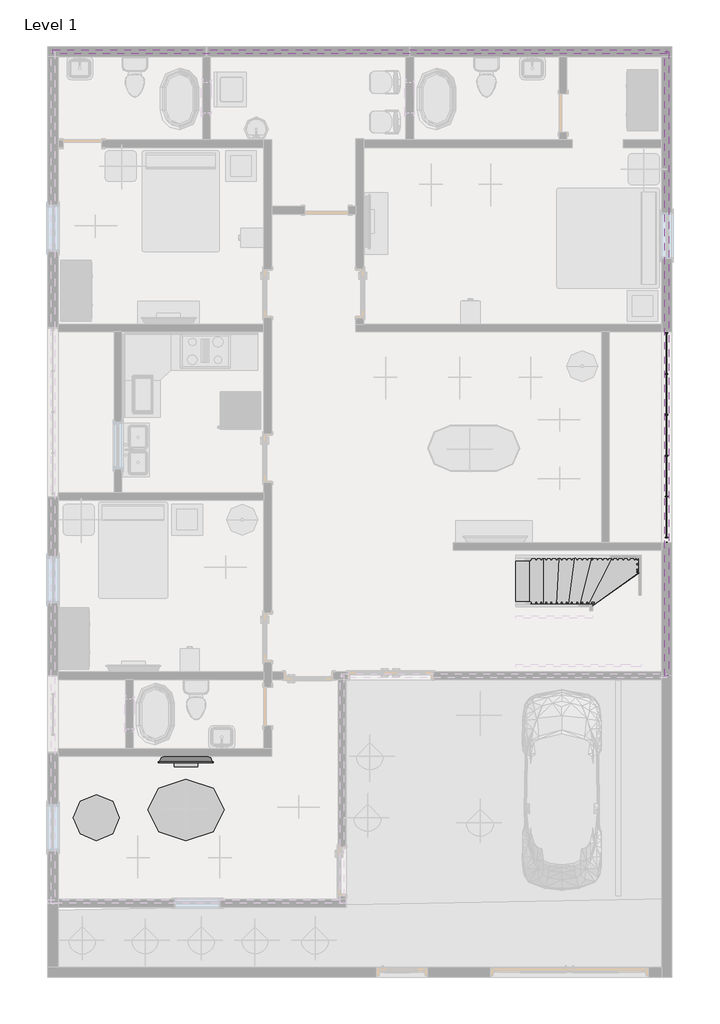
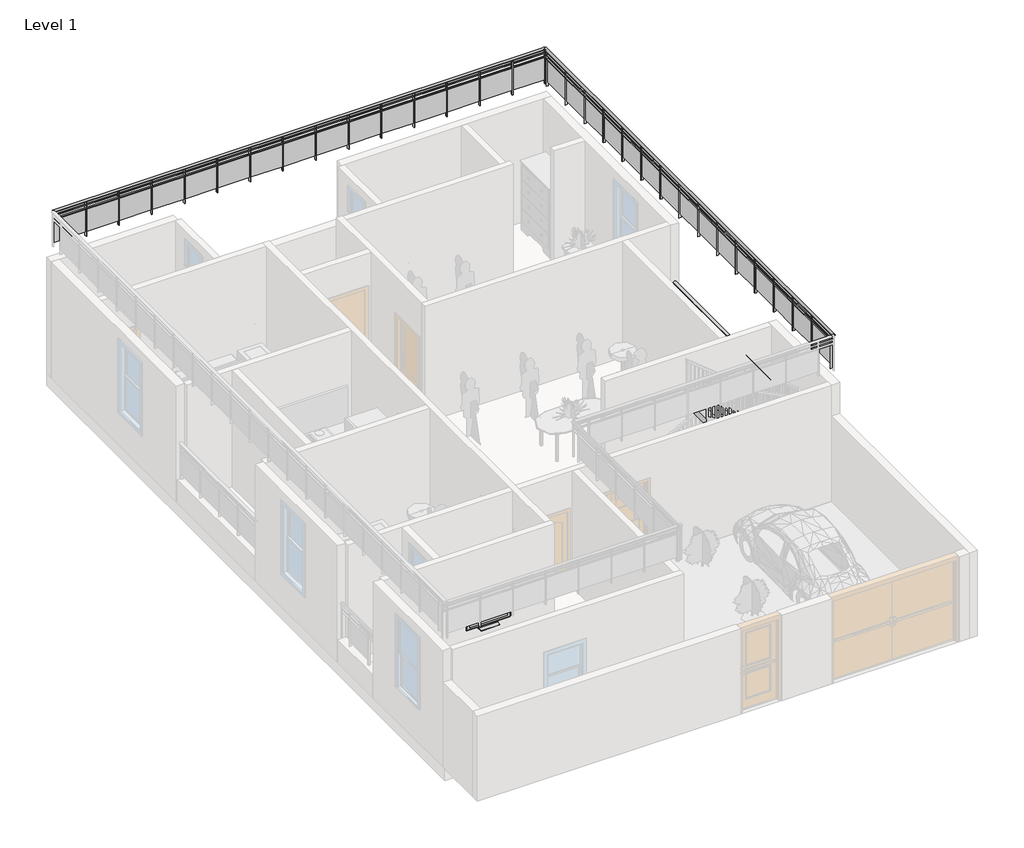
# One storey, part 5 of 6: 3 furniture elements, 3 railings, 1 stair flight.
"""IFC4 building model written with IfcOpenShell, lengths in millimetres."""

from ifc_helpers import new_model, si_unit, point, frame, origin, place, context, project, spatial, polyline, ellipse_curve, trimmed, outline, extrude, transform, mapped, element, save
from ifc_brep_helpers import plane_surface, extruded_surface, advanced_brep
from components import furniture_7a3aaa4f, furniture_905aceb5, furniture_743965d2, stair_flight_813748e6

model = new_model("IFC4")

# Units and contexts
model_context = context("Model", 3, world=origin())
ifc_project = project(units=[si_unit("LENGTHUNIT", "METRE", prefix="MILLI")], contexts=[model_context])

# Site, building, storey
site = spatial("IfcSite", under=ifc_project)
building = spatial("IfcBuilding", under=site)
storey = spatial("IfcBuildingStorey", under=building, Name="Level 1", Elevation=0.0)

# Furniture
placement = place(None, origin())
furniture_shape = furniture_7a3aaa4f(model_context)
element("IfcFurniture", 1, ObjectType="TV - Flat Screen : 42\"", at=placement, inside=storey, context=model_context, shape_type="MappedRepresentation", body=[
    mapped(furniture_shape, transform((-11860.0396044, -302.3114474, 1041.4), x_axis=(1.0, 0.0, 0.0), y_axis=(0.0, 1.0, 0.0), z_axis=(0.0, 0.0, 1.0))),
])
furniture_2_shape = furniture_905aceb5(model_context)
element("IfcFurniture", 2, ObjectType="Table-Dining Round w Chairs : 36\" Diameter", at=placement, inside=storey, context=model_context, shape_type="MappedRepresentation", body=[
    mapped(furniture_2_shape, transform((-13745.6660857, -1278.0941352, 0.0), x_axis=(1.0, 0.0, 0.0), y_axis=(0.0, 1.0, 0.0), z_axis=(0.0, 0.0, 1.0))),
])
furniture_3_shape = furniture_743965d2(model_context)
element("IfcFurniture", 3, ObjectType="Table-Ellipse : 60\" x 48\"", at=placement, inside=storey, context=model_context, shape_type="MappedRepresentation", body=[
    mapped(furniture_3_shape, transform((-11863.9841185, -1310.5728237, 0.0), x_axis=(1.0, 0.0, 0.0), y_axis=(0.0, 1.0, 0.0), z_axis=(0.0, 0.0, 1.0))),
])

# Railings
element("IfcRailing", 4, ObjectType="Glass Panel - Bottom Fill", at=placement, inside=storey, context=model_context, shape_type="SolidModel", body=[
    advanced_brep(
    [(-2351.6841185, 3998.0271763, 1524.0), (-2275.4841185, 3998.0271763, 1524.0), (-2351.6841185, 8265.2271763, 1524.0), (-2275.4841185, 8265.2271763, 1524.0)],
    [
        (0, 1, ellipse_curve(frame((-2313.5841185, 3998.0271763, 1524.0), z_axis=(0.0, -1.0, 0.0), x_axis=(1.0, 0.0, 0.0)), 38.1, 28.575)),
        (1, 0, ellipse_curve(frame((-2313.5841185, 3998.0271763, 1524.0), z_axis=(0.0, -1.0, 0.0), x_axis=(1.0, 0.0, 0.0)), 38.1, 28.575)),
        (2, 3, ellipse_curve(frame((-2313.5841185, 8265.2271763, 1524.0), z_axis=(0.0, 1.0, 0.0), x_axis=(1.0, 0.0, 0.0)), 38.1, 28.575)),
        (3, 2, ellipse_curve(frame((-2313.5841185, 8265.2271763, 1524.0), z_axis=(0.0, 1.0, 0.0), x_axis=(1.0, 0.0, 0.0)), 38.1, 28.575)),
        (0, 2),
        (3, 1),
    ],
    [
        plane_surface(frame((-2313.5841185, 3998.0271763, 1524.0), z_axis=(0.0, -1.0, 0.0), x_axis=(0.0, 0.0, 1.0))),
        plane_surface(frame((-2313.5841185, 8265.2271763, 1524.0), z_axis=(0.0, 1.0, 0.0), x_axis=(0.0, 0.0, 1.0))),
        extruded_surface(trimmed(ellipse_curve(frame((-2313.5841185, 8265.2271763, 1524.0), z_axis=(0.0, -1.0, 0.0), x_axis=(1.0, 0.0, 0.0)), 38.1, 28.575), [point((-2351.6841185, 8265.2271763, 1524.0))], [point((-2275.4841185, 8265.2271763, 1524.0))], True, "CARTESIAN"), (0.0, -4267.200000000001, 0.0), 4267.200000000001),
        extruded_surface(trimmed(ellipse_curve(frame((-2313.5841185, 8265.2271763, 1524.0), z_axis=(0.0, -1.0, 0.0), x_axis=(1.0, 0.0, 0.0)), 38.1, 28.575), [point((-2275.4841185, 8265.2271763, 1524.0))], [point((-2351.6841185, 8265.2271763, 1524.0))], True, "CARTESIAN"), (0.0, -4267.200000000001, 0.0), 4267.200000000001),
    ],
    [
        (0, [[1, 2]]),
        (1, [[3, 4]]),
        (2, [[-1, 5, -4, 6]]),
        (3, [[-2, -6, -3, -5]]),
    ],
),
    extrude(outline(polyline([(-2300.8841185, 3998.0271763), (-2326.2841185, 3998.0271763), (-2326.2841185, 8265.2271763), (-2300.8841185, 8265.2271763), (-2300.8841185, 3998.0271763)])), frame((0.0, 0.0, 1409.7), z_axis=(0.0, 0.0, 1.0), x_axis=(1.0, 0.0, 0.0)), (0.0, 0.0, 1.0), 25.4),
    extrude(outline(polyline([(-2300.8841185, 3998.0271763), (-2326.2841185, 3998.0271763), (-2326.2841185, 8265.2271763), (-2300.8841185, 8265.2271763), (-2300.8841185, 3998.0271763)])), frame((0.0, 0.0, 1308.1), z_axis=(0.0, 0.0, 1.0), x_axis=(1.0, 0.0, 0.0)), (0.0, 0.0, 1.0), 25.4),
    extrude(outline(polyline([(-2288.1841185, 8157.2771763), (-2338.9841185, 8157.2771763), (-2338.9841185, 8169.9771763), (-2288.1841185, 8169.9771763), (-2288.1841185, 8157.2771763)])), frame((0.0, 0.0, 609.6), z_axis=(0.0, 0.0, 1.0), x_axis=(1.0, 0.0, 0.0)), (0.0, 0.0, 1.0), 885.6788223),
    extrude(outline(polyline([(-2320.1192755, 7350.8271763), (-2320.1192755, 8163.6271763), (-2313.7692755, 8163.6271763), (-2313.7692755, 7350.8271763), (-2320.1192755, 7350.8271763)])), frame((0.0, 0.0, 711.2), z_axis=(0.0, 0.0, 1.0), x_axis=(1.0, 0.0, 0.0)), (0.0, 0.0, 1.0), 596.9),
    extrude(outline(polyline([(-2288.1841185, 7344.4771763), (-2338.9841185, 7344.4771763), (-2338.9841185, 7357.1771763), (-2288.1841185, 7357.1771763), (-2288.1841185, 7344.4771763)])), frame((0.0, 0.0, 609.6), z_axis=(0.0, 0.0, 1.0), x_axis=(1.0, 0.0, 0.0)), (0.0, 0.0, 1.0), 885.6788223),
    extrude(outline(polyline([(-2320.1192755, 6538.0271763), (-2320.1192755, 7350.8271763), (-2313.7692755, 7350.8271763), (-2313.7692755, 6538.0271763), (-2320.1192755, 6538.0271763)])), frame((0.0, 0.0, 711.2), z_axis=(0.0, 0.0, 1.0), x_axis=(1.0, 0.0, 0.0)), (0.0, 0.0, 1.0), 596.9),
    extrude(outline(polyline([(-2288.1841185, 6531.6771763), (-2338.9841185, 6531.6771763), (-2338.9841185, 6544.3771763), (-2288.1841185, 6544.3771763), (-2288.1841185, 6531.6771763)])), frame((0.0, 0.0, 609.6), z_axis=(0.0, 0.0, 1.0), x_axis=(1.0, 0.0, 0.0)), (0.0, 0.0, 1.0), 885.6788223),
    extrude(outline(polyline([(-2320.1192755, 5725.2271763), (-2320.1192755, 6538.0271763), (-2313.7692755, 6538.0271763), (-2313.7692755, 5725.2271763), (-2320.1192755, 5725.2271763)])), frame((0.0, 0.0, 711.2), z_axis=(0.0, 0.0, 1.0), x_axis=(1.0, 0.0, 0.0)), (0.0, 0.0, 1.0), 596.9),
    extrude(outline(polyline([(-2288.1841185, 5718.8771763), (-2338.9841185, 5718.8771763), (-2338.9841185, 5731.5771763), (-2288.1841185, 5731.5771763), (-2288.1841185, 5718.8771763)])), frame((0.0, 0.0, 609.6), z_axis=(0.0, 0.0, 1.0), x_axis=(1.0, 0.0, 0.0)), (0.0, 0.0, 1.0), 885.6788223),
    extrude(outline(polyline([(-2320.1192755, 4912.4271763), (-2320.1192755, 5725.2271763), (-2313.7692755, 5725.2271763), (-2313.7692755, 4912.4271763), (-2320.1192755, 4912.4271763)])), frame((0.0, 0.0, 711.2), z_axis=(0.0, 0.0, 1.0), x_axis=(1.0, 0.0, 0.0)), (0.0, 0.0, 1.0), 596.9),
    extrude(outline(polyline([(-2288.1841185, 4906.0771763), (-2338.9841185, 4906.0771763), (-2338.9841185, 4918.7771763), (-2288.1841185, 4918.7771763), (-2288.1841185, 4906.0771763)])), frame((0.0, 0.0, 609.6), z_axis=(0.0, 0.0, 1.0), x_axis=(1.0, 0.0, 0.0)), (0.0, 0.0, 1.0), 885.6788223),
    extrude(outline(polyline([(-2320.1192755, 4099.6271763), (-2320.1192755, 4912.4271763), (-2313.7692755, 4912.4271763), (-2313.7692755, 4099.6271763), (-2320.1192755, 4099.6271763)])), frame((0.0, 0.0, 711.2), z_axis=(0.0, 0.0, 1.0), x_axis=(1.0, 0.0, 0.0)), (0.0, 0.0, 1.0), 596.9),
    extrude(outline(polyline([(-2288.1841185, 4093.2771763), (-2338.9841185, 4093.2771763), (-2338.9841185, 4105.9771763), (-2288.1841185, 4105.9771763), (-2288.1841185, 4093.2771763)])), frame((0.0, 0.0, 609.6), z_axis=(0.0, 0.0, 1.0), x_axis=(1.0, 0.0, 0.0)), (0.0, 0.0, 1.0), 885.6788223),
    extrude(outline(polyline([(-2304.0591185, 8252.5271763), (-2323.1091185, 8252.5271763), (-2323.1091185, 8271.5771763), (-2304.0591185, 8271.5771763), (-2304.0591185, 8252.5271763)])), frame((0.0, 0.0, 609.6), z_axis=(0.0, 0.0, 1.0), x_axis=(1.0, 0.0, 0.0)), (0.0, 0.0, 1.0), 885.6788223),
    extrude(outline(polyline([(-2304.0591185, 3991.6771763), (-2323.1091185, 3991.6771763), (-2323.1091185, 4010.7271763), (-2304.0591185, 4010.7271763), (-2304.0591185, 3991.6771763)])), frame((0.0, 0.0, 609.6), z_axis=(0.0, 0.0, 1.0), x_axis=(1.0, 0.0, 0.0)), (0.0, 0.0, 1.0), 885.6788223),
])
element("IfcRailing", 5, ObjectType="Glass Panel - Bottom Fill", at=placement, inside=storey, context=model_context, shape_type="SolidModel", body=[
    advanced_brep(
    [(-14505.5841185, 13789.7271763, 4267.2), (-14505.5841185, 13713.5271763, 4267.2), (-2313.5841185, 13789.7271763, 4267.2), (-2313.5841185, 13713.5271763, 4267.2)],
    [
        (0, 1, ellipse_curve(frame((-14505.5841185, 13751.6271763, 4267.2), z_axis=(-1.0, 0.0, 0.0), x_axis=(0.0, -1.0, 0.0)), 38.1, 28.575)),
        (1, 0, ellipse_curve(frame((-14505.5841185, 13751.6271763, 4267.2), z_axis=(-1.0, 0.0, 0.0), x_axis=(0.0, -1.0, 0.0)), 38.1, 28.575)),
        (2, 3, ellipse_curve(frame((-2313.5841185, 13751.6271763, 4267.2), z_axis=(1.0, 0.0, 0.0), x_axis=(0.0, -1.0, 0.0)), 38.1, 28.575)),
        (3, 2, ellipse_curve(frame((-2313.5841185, 13751.6271763, 4267.2), z_axis=(1.0, 0.0, 0.0), x_axis=(0.0, -1.0, 0.0)), 38.1, 28.575)),
        (0, 2),
        (3, 1),
    ],
    [
        plane_surface(frame((-14505.5841185, 13751.6271763, 4267.2), z_axis=(-1.0, 0.0, 0.0), x_axis=(0.0, 1.0, 0.0))),
        plane_surface(frame((-2313.5841185, 13751.6271763, 4267.2), z_axis=(1.0, 0.0, 0.0), x_axis=(0.0, 1.0, 0.0))),
        extruded_surface(trimmed(ellipse_curve(frame((-2313.5841185, 13751.6271763, 4267.2), z_axis=(-1.0, 0.0, 0.0), x_axis=(0.0, -1.0, 0.0)), 38.1, 28.575), [point((-2313.5841185, 13789.7271763, 4267.2))], [point((-2313.5841185, 13713.5271763, 4267.2))], True, "CARTESIAN"), (-12192.0, 0.0, 0.0), 12192.0),
        extruded_surface(trimmed(ellipse_curve(frame((-2313.5841185, 13751.6271763, 4267.2), z_axis=(-1.0, 0.0, 0.0), x_axis=(0.0, -1.0, 0.0)), 38.1, 28.575), [point((-2313.5841185, 13713.5271763, 4267.2))], [point((-2313.5841185, 13789.7271763, 4267.2))], True, "CARTESIAN"), (-12192.0, 0.0, 0.0), 12192.0),
    ],
    [
        (0, [[1, 2]]),
        (1, [[3, 4]]),
        (2, [[-1, 5, -4, 6]]),
        (3, [[-2, -6, -3, -5]]),
    ],
),
    extrude(outline(polyline([(-14505.5841185, 13738.9271763), (-14505.5841185, 13764.3271763), (-2313.5841185, 13764.3271763), (-2313.5841185, 13738.9271763), (-14505.5841185, 13738.9271763)])), frame((0.0, 0.0, 4152.9), z_axis=(0.0, 0.0, 1.0), x_axis=(1.0, 0.0, 0.0)), (0.0, 0.0, 1.0), 25.4),
    extrude(outline(polyline([(-14505.5841185, 13738.9271763), (-14505.5841185, 13764.3271763), (-2313.5841185, 13764.3271763), (-2313.5841185, 13738.9271763), (-14505.5841185, 13738.9271763)])), frame((0.0, 0.0, 4051.3), z_axis=(0.0, 0.0, 1.0), x_axis=(1.0, 0.0, 0.0)), (0.0, 0.0, 1.0), 25.4),
    extrude(outline(polyline([(-3126.3841185, 13758.1623333), (-2313.5841185, 13758.1623333), (-2313.5841185, 13751.8123333), (-3126.3841185, 13751.8123333), (-3126.3841185, 13758.1623333)])), frame((0.0, 0.0, 3454.4), z_axis=(0.0, 0.0, 1.0), x_axis=(1.0, 0.0, 0.0)), (0.0, 0.0, 1.0), 596.9),
    extrude(outline(polyline([(-3132.7341185, 13726.2271763), (-3132.7341185, 13777.0271763), (-3120.0341185, 13777.0271763), (-3120.0341185, 13726.2271763), (-3132.7341185, 13726.2271763)])), frame((0.0, 0.0, 3352.8), z_axis=(0.0, 0.0, 1.0), x_axis=(1.0, 0.0, 0.0)), (0.0, 0.0, 1.0), 885.6788223),
    extrude(outline(polyline([(-3939.1841185, 13758.1623333), (-3126.3841185, 13758.1623333), (-3126.3841185, 13751.8123333), (-3939.1841185, 13751.8123333), (-3939.1841185, 13758.1623333)])), frame((0.0, 0.0, 3454.4), z_axis=(0.0, 0.0, 1.0), x_axis=(1.0, 0.0, 0.0)), (0.0, 0.0, 1.0), 596.9),
    extrude(outline(polyline([(-3945.5341185, 13726.2271763), (-3945.5341185, 13777.0271763), (-3932.8341185, 13777.0271763), (-3932.8341185, 13726.2271763), (-3945.5341185, 13726.2271763)])), frame((0.0, 0.0, 3352.8), z_axis=(0.0, 0.0, 1.0), x_axis=(1.0, 0.0, 0.0)), (0.0, 0.0, 1.0), 885.6788223),
    extrude(outline(polyline([(-4751.9841185, 13758.1623333), (-3939.1841185, 13758.1623333), (-3939.1841185, 13751.8123333), (-4751.9841185, 13751.8123333), (-4751.9841185, 13758.1623333)])), frame((0.0, 0.0, 3454.4), z_axis=(0.0, 0.0, 1.0), x_axis=(1.0, 0.0, 0.0)), (0.0, 0.0, 1.0), 596.9),
    extrude(outline(polyline([(-4758.3341185, 13726.2271763), (-4758.3341185, 13777.0271763), (-4745.6341185, 13777.0271763), (-4745.6341185, 13726.2271763), (-4758.3341185, 13726.2271763)])), frame((0.0, 0.0, 3352.8), z_axis=(0.0, 0.0, 1.0), x_axis=(1.0, 0.0, 0.0)), (0.0, 0.0, 1.0), 885.6788223),
    extrude(outline(polyline([(-5564.7841185, 13758.1623333), (-4751.9841185, 13758.1623333), (-4751.9841185, 13751.8123333), (-5564.7841185, 13751.8123333), (-5564.7841185, 13758.1623333)])), frame((0.0, 0.0, 3454.4), z_axis=(0.0, 0.0, 1.0), x_axis=(1.0, 0.0, 0.0)), (0.0, 0.0, 1.0), 596.9),
    extrude(outline(polyline([(-5571.1341185, 13726.2271763), (-5571.1341185, 13777.0271763), (-5558.4341185, 13777.0271763), (-5558.4341185, 13726.2271763), (-5571.1341185, 13726.2271763)])), frame((0.0, 0.0, 3352.8), z_axis=(0.0, 0.0, 1.0), x_axis=(1.0, 0.0, 0.0)), (0.0, 0.0, 1.0), 885.6788223),
    extrude(outline(polyline([(-6377.5841185, 13758.1623333), (-5564.7841185, 13758.1623333), (-5564.7841185, 13751.8123333), (-6377.5841185, 13751.8123333), (-6377.5841185, 13758.1623333)])), frame((0.0, 0.0, 3454.4), z_axis=(0.0, 0.0, 1.0), x_axis=(1.0, 0.0, 0.0)), (0.0, 0.0, 1.0), 596.9),
    extrude(outline(polyline([(-6383.9341185, 13726.2271763), (-6383.9341185, 13777.0271763), (-6371.2341185, 13777.0271763), (-6371.2341185, 13726.2271763), (-6383.9341185, 13726.2271763)])), frame((0.0, 0.0, 3352.8), z_axis=(0.0, 0.0, 1.0), x_axis=(1.0, 0.0, 0.0)), (0.0, 0.0, 1.0), 885.6788223),
    extrude(outline(polyline([(-7190.3841185, 13758.1623333), (-6377.5841185, 13758.1623333), (-6377.5841185, 13751.8123333), (-7190.3841185, 13751.8123333), (-7190.3841185, 13758.1623333)])), frame((0.0, 0.0, 3454.4), z_axis=(0.0, 0.0, 1.0), x_axis=(1.0, 0.0, 0.0)), (0.0, 0.0, 1.0), 596.9),
    extrude(outline(polyline([(-7196.7341185, 13726.2271763), (-7196.7341185, 13777.0271763), (-7184.0341185, 13777.0271763), (-7184.0341185, 13726.2271763), (-7196.7341185, 13726.2271763)])), frame((0.0, 0.0, 3352.8), z_axis=(0.0, 0.0, 1.0), x_axis=(1.0, 0.0, 0.0)), (0.0, 0.0, 1.0), 885.6788223),
    extrude(outline(polyline([(-8003.1841185, 13758.1623333), (-7190.3841185, 13758.1623333), (-7190.3841185, 13751.8123333), (-8003.1841185, 13751.8123333), (-8003.1841185, 13758.1623333)])), frame((0.0, 0.0, 3454.4), z_axis=(0.0, 0.0, 1.0), x_axis=(1.0, 0.0, 0.0)), (0.0, 0.0, 1.0), 596.9),
    extrude(outline(polyline([(-8009.5341185, 13726.2271763), (-8009.5341185, 13777.0271763), (-7996.8341185, 13777.0271763), (-7996.8341185, 13726.2271763), (-8009.5341185, 13726.2271763)])), frame((0.0, 0.0, 3352.8), z_axis=(0.0, 0.0, 1.0), x_axis=(1.0, 0.0, 0.0)), (0.0, 0.0, 1.0), 885.6788223),
    extrude(outline(polyline([(-8815.9841185, 13758.1623333), (-8003.1841185, 13758.1623333), (-8003.1841185, 13751.8123333), (-8815.9841185, 13751.8123333), (-8815.9841185, 13758.1623333)])), frame((0.0, 0.0, 3454.4), z_axis=(0.0, 0.0, 1.0), x_axis=(1.0, 0.0, 0.0)), (0.0, 0.0, 1.0), 596.9),
    extrude(outline(polyline([(-8822.3341185, 13726.2271763), (-8822.3341185, 13777.0271763), (-8809.6341185, 13777.0271763), (-8809.6341185, 13726.2271763), (-8822.3341185, 13726.2271763)])), frame((0.0, 0.0, 3352.8), z_axis=(0.0, 0.0, 1.0), x_axis=(1.0, 0.0, 0.0)), (0.0, 0.0, 1.0), 885.6788223),
    extrude(outline(polyline([(-9628.7841185, 13758.1623333), (-8815.9841185, 13758.1623333), (-8815.9841185, 13751.8123333), (-9628.7841185, 13751.8123333), (-9628.7841185, 13758.1623333)])), frame((0.0, 0.0, 3454.4), z_axis=(0.0, 0.0, 1.0), x_axis=(1.0, 0.0, 0.0)), (0.0, 0.0, 1.0), 596.9),
    extrude(outline(polyline([(-9635.1341185, 13726.2271763), (-9635.1341185, 13777.0271763), (-9622.4341185, 13777.0271763), (-9622.4341185, 13726.2271763), (-9635.1341185, 13726.2271763)])), frame((0.0, 0.0, 3352.8), z_axis=(0.0, 0.0, 1.0), x_axis=(1.0, 0.0, 0.0)), (0.0, 0.0, 1.0), 885.6788223),
    extrude(outline(polyline([(-10441.5841185, 13758.1623333), (-9628.7841185, 13758.1623333), (-9628.7841185, 13751.8123333), (-10441.5841185, 13751.8123333), (-10441.5841185, 13758.1623333)])), frame((0.0, 0.0, 3454.4), z_axis=(0.0, 0.0, 1.0), x_axis=(1.0, 0.0, 0.0)), (0.0, 0.0, 1.0), 596.9),
    extrude(outline(polyline([(-10447.9341185, 13726.2271763), (-10447.9341185, 13777.0271763), (-10435.2341185, 13777.0271763), (-10435.2341185, 13726.2271763), (-10447.9341185, 13726.2271763)])), frame((0.0, 0.0, 3352.8), z_axis=(0.0, 0.0, 1.0), x_axis=(1.0, 0.0, 0.0)), (0.0, 0.0, 1.0), 885.6788223),
    extrude(outline(polyline([(-11254.3841185, 13758.1623333), (-10441.5841185, 13758.1623333), (-10441.5841185, 13751.8123333), (-11254.3841185, 13751.8123333), (-11254.3841185, 13758.1623333)])), frame((0.0, 0.0, 3454.4), z_axis=(0.0, 0.0, 1.0), x_axis=(1.0, 0.0, 0.0)), (0.0, 0.0, 1.0), 596.9),
    extrude(outline(polyline([(-11260.7341185, 13726.2271763), (-11260.7341185, 13777.0271763), (-11248.0341185, 13777.0271763), (-11248.0341185, 13726.2271763), (-11260.7341185, 13726.2271763)])), frame((0.0, 0.0, 3352.8), z_axis=(0.0, 0.0, 1.0), x_axis=(1.0, 0.0, 0.0)), (0.0, 0.0, 1.0), 885.6788223),
    extrude(outline(polyline([(-12067.1841185, 13758.1623333), (-11254.3841185, 13758.1623333), (-11254.3841185, 13751.8123333), (-12067.1841185, 13751.8123333), (-12067.1841185, 13758.1623333)])), frame((0.0, 0.0, 3454.4), z_axis=(0.0, 0.0, 1.0), x_axis=(1.0, 0.0, 0.0)), (0.0, 0.0, 1.0), 596.9),
    extrude(outline(polyline([(-12073.5341185, 13726.2271763), (-12073.5341185, 13777.0271763), (-12060.8341185, 13777.0271763), (-12060.8341185, 13726.2271763), (-12073.5341185, 13726.2271763)])), frame((0.0, 0.0, 3352.8), z_axis=(0.0, 0.0, 1.0), x_axis=(1.0, 0.0, 0.0)), (0.0, 0.0, 1.0), 885.6788223),
    extrude(outline(polyline([(-12879.9841185, 13758.1623333), (-12067.1841185, 13758.1623333), (-12067.1841185, 13751.8123333), (-12879.9841185, 13751.8123333), (-12879.9841185, 13758.1623333)])), frame((0.0, 0.0, 3454.4), z_axis=(0.0, 0.0, 1.0), x_axis=(1.0, 0.0, 0.0)), (0.0, 0.0, 1.0), 596.9),
    extrude(outline(polyline([(-12886.3341185, 13726.2271763), (-12886.3341185, 13777.0271763), (-12873.6341185, 13777.0271763), (-12873.6341185, 13726.2271763), (-12886.3341185, 13726.2271763)])), frame((0.0, 0.0, 3352.8), z_axis=(0.0, 0.0, 1.0), x_axis=(1.0, 0.0, 0.0)), (0.0, 0.0, 1.0), 885.6788223),
    extrude(outline(polyline([(-13692.7841185, 13758.1623333), (-12879.9841185, 13758.1623333), (-12879.9841185, 13751.8123333), (-13692.7841185, 13751.8123333), (-13692.7841185, 13758.1623333)])), frame((0.0, 0.0, 3454.4), z_axis=(0.0, 0.0, 1.0), x_axis=(1.0, 0.0, 0.0)), (0.0, 0.0, 1.0), 596.9),
    extrude(outline(polyline([(-13699.1341185, 13726.2271763), (-13699.1341185, 13777.0271763), (-13686.4341185, 13777.0271763), (-13686.4341185, 13726.2271763), (-13699.1341185, 13726.2271763)])), frame((0.0, 0.0, 3352.8), z_axis=(0.0, 0.0, 1.0), x_axis=(1.0, 0.0, 0.0)), (0.0, 0.0, 1.0), 885.6788223),
    extrude(outline(polyline([(-14505.5841185, 13758.1623333), (-13692.7841185, 13758.1623333), (-13692.7841185, 13751.8123333), (-14505.5841185, 13751.8123333), (-14505.5841185, 13758.1623333)])), frame((0.0, 0.0, 3454.4), z_axis=(0.0, 0.0, 1.0), x_axis=(1.0, 0.0, 0.0)), (0.0, 0.0, 1.0), 596.9),
    extrude(outline(polyline([(-2326.2841185, 13742.1021763), (-2326.2841185, 13761.1521763), (-2307.2341185, 13761.1521763), (-2307.2341185, 13742.1021763), (-2326.2841185, 13742.1021763)])), frame((0.0, 0.0, 3352.8), z_axis=(0.0, 0.0, 1.0), x_axis=(1.0, 0.0, 0.0)), (0.0, 0.0, 1.0), 885.6788223),
    extrude(outline(polyline([(-14511.9341185, 13742.1021763), (-14511.9341185, 13761.1521763), (-14492.8841185, 13761.1521763), (-14492.8841185, 13742.1021763), (-14511.9341185, 13742.1021763)])), frame((0.0, 0.0, 3352.8), z_axis=(0.0, 0.0, 1.0), x_axis=(1.0, 0.0, 0.0)), (0.0, 0.0, 1.0), 885.6788223),
])
element("IfcRailing", 6, ObjectType="Glass Panel - Bottom Fill", at=placement, inside=storey, context=model_context, shape_type="SolidModel", body=[
    advanced_brep(
    [(-2275.4841185, 13751.6271763, 4267.2), (-2351.6841185, 13751.6271763, 4267.2), (-2275.4841185, 1356.4271763, 4267.2), (-2351.6841185, 1356.4271763, 4267.2)],
    [
        (0, 1, ellipse_curve(frame((-2313.5841185, 13751.6271763, 4267.2), z_axis=(0.0, 1.0, 0.0), x_axis=(-1.0, 0.0, 0.0)), 38.1, 28.575)),
        (1, 0, ellipse_curve(frame((-2313.5841185, 13751.6271763, 4267.2), z_axis=(0.0, 1.0, 0.0), x_axis=(-1.0, 0.0, 0.0)), 38.1, 28.575)),
        (2, 3, ellipse_curve(frame((-2313.5841185, 1356.4271763, 4267.2), z_axis=(0.0, -1.0, 0.0), x_axis=(-1.0, 0.0, 0.0)), 38.1, 28.575)),
        (3, 2, ellipse_curve(frame((-2313.5841185, 1356.4271763, 4267.2), z_axis=(0.0, -1.0, 0.0), x_axis=(-1.0, 0.0, 0.0)), 38.1, 28.575)),
        (0, 2),
        (3, 1),
    ],
    [
        plane_surface(frame((-2313.5841185, 13751.6271763, 4267.2), z_axis=(0.0, 1.0, 0.0), x_axis=(0.0, 0.0, -1.0))),
        plane_surface(frame((-2313.5841185, 1356.4271763, 4267.2), z_axis=(0.0, -1.0, 0.0), x_axis=(0.0, 0.0, -1.0))),
        extruded_surface(trimmed(ellipse_curve(frame((-2313.5841185, 1356.4271763, 4267.2), z_axis=(0.0, 1.0, 0.0), x_axis=(-1.0, 0.0, 0.0)), 38.1, 28.575), [point((-2275.4841185, 1356.4271763, 4267.2))], [point((-2351.6841185, 1356.4271763, 4267.2))], True, "CARTESIAN"), (0.0, 12395.2, 0.0), 12395.2),
        extruded_surface(trimmed(ellipse_curve(frame((-2313.5841185, 1356.4271763, 4267.2), z_axis=(0.0, 1.0, 0.0), x_axis=(-1.0, 0.0, 0.0)), 38.1, 28.575), [point((-2351.6841185, 1356.4271763, 4267.2))], [point((-2275.4841185, 1356.4271763, 4267.2))], True, "CARTESIAN"), (0.0, 12395.2, 0.0), 12395.2),
    ],
    [
        (0, [[1, 2]]),
        (1, [[3, 4]]),
        (2, [[-1, 5, -4, 6]]),
        (3, [[-2, -6, -3, -5]]),
    ],
),
    extrude(outline(polyline([(-2326.2841185, 13751.6271763), (-2300.8841185, 13751.6271763), (-2300.8841185, 1356.4271763), (-2326.2841185, 1356.4271763), (-2326.2841185, 13751.6271763)])), frame((0.0, 0.0, 4152.9), z_axis=(0.0, 0.0, 1.0), x_axis=(1.0, 0.0, 0.0)), (0.0, 0.0, 1.0), 25.4),
    extrude(outline(polyline([(-2326.2841185, 13751.6271763), (-2300.8841185, 13751.6271763), (-2300.8841185, 1356.4271763), (-2326.2841185, 1356.4271763), (-2326.2841185, 13751.6271763)])), frame((0.0, 0.0, 4051.3), z_axis=(0.0, 0.0, 1.0), x_axis=(1.0, 0.0, 0.0)), (0.0, 0.0, 1.0), 25.4),
    extrude(outline(polyline([(-2338.9841185, 1464.3771763), (-2288.1841185, 1464.3771763), (-2288.1841185, 1451.6771763), (-2338.9841185, 1451.6771763), (-2338.9841185, 1464.3771763)])), frame((0.0, 0.0, 3352.8), z_axis=(0.0, 0.0, 1.0), x_axis=(1.0, 0.0, 0.0)), (0.0, 0.0, 1.0), 885.6788223),
    extrude(outline(polyline([(-2307.0489615, 2270.8271763), (-2307.0489615, 1458.0271763), (-2313.3989615, 1458.0271763), (-2313.3989615, 2270.8271763), (-2307.0489615, 2270.8271763)])), frame((0.0, 0.0, 3454.4), z_axis=(0.0, 0.0, 1.0), x_axis=(1.0, 0.0, 0.0)), (0.0, 0.0, 1.0), 596.9),
    extrude(outline(polyline([(-2338.9841185, 2277.1771763), (-2288.1841185, 2277.1771763), (-2288.1841185, 2264.4771763), (-2338.9841185, 2264.4771763), (-2338.9841185, 2277.1771763)])), frame((0.0, 0.0, 3352.8), z_axis=(0.0, 0.0, 1.0), x_axis=(1.0, 0.0, 0.0)), (0.0, 0.0, 1.0), 885.6788223),
    extrude(outline(polyline([(-2307.0489615, 3083.6271763), (-2307.0489615, 2270.8271763), (-2313.3989615, 2270.8271763), (-2313.3989615, 3083.6271763), (-2307.0489615, 3083.6271763)])), frame((0.0, 0.0, 3454.4), z_axis=(0.0, 0.0, 1.0), x_axis=(1.0, 0.0, 0.0)), (0.0, 0.0, 1.0), 596.9),
    extrude(outline(polyline([(-2338.9841185, 3089.9771763), (-2288.1841185, 3089.9771763), (-2288.1841185, 3077.2771763), (-2338.9841185, 3077.2771763), (-2338.9841185, 3089.9771763)])), frame((0.0, 0.0, 3352.8), z_axis=(0.0, 0.0, 1.0), x_axis=(1.0, 0.0, 0.0)), (0.0, 0.0, 1.0), 885.6788223),
    extrude(outline(polyline([(-2307.0489615, 3896.4271763), (-2307.0489615, 3083.6271763), (-2313.3989615, 3083.6271763), (-2313.3989615, 3896.4271763), (-2307.0489615, 3896.4271763)])), frame((0.0, 0.0, 3454.4), z_axis=(0.0, 0.0, 1.0), x_axis=(1.0, 0.0, 0.0)), (0.0, 0.0, 1.0), 596.9),
    extrude(outline(polyline([(-2338.9841185, 3902.7771763), (-2288.1841185, 3902.7771763), (-2288.1841185, 3890.0771763), (-2338.9841185, 3890.0771763), (-2338.9841185, 3902.7771763)])), frame((0.0, 0.0, 3352.8), z_axis=(0.0, 0.0, 1.0), x_axis=(1.0, 0.0, 0.0)), (0.0, 0.0, 1.0), 885.6788223),
    extrude(outline(polyline([(-2307.0489615, 4709.2271763), (-2307.0489615, 3896.4271763), (-2313.3989615, 3896.4271763), (-2313.3989615, 4709.2271763), (-2307.0489615, 4709.2271763)])), frame((0.0, 0.0, 3454.4), z_axis=(0.0, 0.0, 1.0), x_axis=(1.0, 0.0, 0.0)), (0.0, 0.0, 1.0), 596.9),
    extrude(outline(polyline([(-2338.9841185, 4715.5771763), (-2288.1841185, 4715.5771763), (-2288.1841185, 4702.8771763), (-2338.9841185, 4702.8771763), (-2338.9841185, 4715.5771763)])), frame((0.0, 0.0, 3352.8), z_axis=(0.0, 0.0, 1.0), x_axis=(1.0, 0.0, 0.0)), (0.0, 0.0, 1.0), 885.6788223),
    extrude(outline(polyline([(-2307.0489615, 5522.0271763), (-2307.0489615, 4709.2271763), (-2313.3989615, 4709.2271763), (-2313.3989615, 5522.0271763), (-2307.0489615, 5522.0271763)])), frame((0.0, 0.0, 3454.4), z_axis=(0.0, 0.0, 1.0), x_axis=(1.0, 0.0, 0.0)), (0.0, 0.0, 1.0), 596.9),
    extrude(outline(polyline([(-2338.9841185, 5528.3771763), (-2288.1841185, 5528.3771763), (-2288.1841185, 5515.6771763), (-2338.9841185, 5515.6771763), (-2338.9841185, 5528.3771763)])), frame((0.0, 0.0, 3352.8), z_axis=(0.0, 0.0, 1.0), x_axis=(1.0, 0.0, 0.0)), (0.0, 0.0, 1.0), 885.6788223),
    extrude(outline(polyline([(-2307.0489615, 6334.8271763), (-2307.0489615, 5522.0271763), (-2313.3989615, 5522.0271763), (-2313.3989615, 6334.8271763), (-2307.0489615, 6334.8271763)])), frame((0.0, 0.0, 3454.4), z_axis=(0.0, 0.0, 1.0), x_axis=(1.0, 0.0, 0.0)), (0.0, 0.0, 1.0), 596.9),
    extrude(outline(polyline([(-2338.9841185, 6341.1771763), (-2288.1841185, 6341.1771763), (-2288.1841185, 6328.4771763), (-2338.9841185, 6328.4771763), (-2338.9841185, 6341.1771763)])), frame((0.0, 0.0, 3352.8), z_axis=(0.0, 0.0, 1.0), x_axis=(1.0, 0.0, 0.0)), (0.0, 0.0, 1.0), 885.6788223),
    extrude(outline(polyline([(-2307.0489615, 7147.6271763), (-2307.0489615, 6334.8271763), (-2313.3989615, 6334.8271763), (-2313.3989615, 7147.6271763), (-2307.0489615, 7147.6271763)])), frame((0.0, 0.0, 3454.4), z_axis=(0.0, 0.0, 1.0), x_axis=(1.0, 0.0, 0.0)), (0.0, 0.0, 1.0), 596.9),
    extrude(outline(polyline([(-2338.9841185, 7153.9771763), (-2288.1841185, 7153.9771763), (-2288.1841185, 7141.2771763), (-2338.9841185, 7141.2771763), (-2338.9841185, 7153.9771763)])), frame((0.0, 0.0, 3352.8), z_axis=(0.0, 0.0, 1.0), x_axis=(1.0, 0.0, 0.0)), (0.0, 0.0, 1.0), 885.6788223),
    extrude(outline(polyline([(-2307.0489615, 7960.4271763), (-2307.0489615, 7147.6271763), (-2313.3989615, 7147.6271763), (-2313.3989615, 7960.4271763), (-2307.0489615, 7960.4271763)])), frame((0.0, 0.0, 3454.4), z_axis=(0.0, 0.0, 1.0), x_axis=(1.0, 0.0, 0.0)), (0.0, 0.0, 1.0), 596.9),
    extrude(outline(polyline([(-2338.9841185, 7966.7771763), (-2288.1841185, 7966.7771763), (-2288.1841185, 7954.0771763), (-2338.9841185, 7954.0771763), (-2338.9841185, 7966.7771763)])), frame((0.0, 0.0, 3352.8), z_axis=(0.0, 0.0, 1.0), x_axis=(1.0, 0.0, 0.0)), (0.0, 0.0, 1.0), 885.6788223),
    extrude(outline(polyline([(-2307.0489615, 8773.2271763), (-2307.0489615, 7960.4271763), (-2313.3989615, 7960.4271763), (-2313.3989615, 8773.2271763), (-2307.0489615, 8773.2271763)])), frame((0.0, 0.0, 3454.4), z_axis=(0.0, 0.0, 1.0), x_axis=(1.0, 0.0, 0.0)), (0.0, 0.0, 1.0), 596.9),
    extrude(outline(polyline([(-2338.9841185, 8779.5771763), (-2288.1841185, 8779.5771763), (-2288.1841185, 8766.8771763), (-2338.9841185, 8766.8771763), (-2338.9841185, 8779.5771763)])), frame((0.0, 0.0, 3352.8), z_axis=(0.0, 0.0, 1.0), x_axis=(1.0, 0.0, 0.0)), (0.0, 0.0, 1.0), 885.6788223),
    extrude(outline(polyline([(-2307.0489615, 9586.0271763), (-2307.0489615, 8773.2271763), (-2313.3989615, 8773.2271763), (-2313.3989615, 9586.0271763), (-2307.0489615, 9586.0271763)])), frame((0.0, 0.0, 3454.4), z_axis=(0.0, 0.0, 1.0), x_axis=(1.0, 0.0, 0.0)), (0.0, 0.0, 1.0), 596.9),
    extrude(outline(polyline([(-2338.9841185, 9592.3771763), (-2288.1841185, 9592.3771763), (-2288.1841185, 9579.6771763), (-2338.9841185, 9579.6771763), (-2338.9841185, 9592.3771763)])), frame((0.0, 0.0, 3352.8), z_axis=(0.0, 0.0, 1.0), x_axis=(1.0, 0.0, 0.0)), (0.0, 0.0, 1.0), 885.6788223),
    extrude(outline(polyline([(-2307.0489615, 10398.8271763), (-2307.0489615, 9586.0271763), (-2313.3989615, 9586.0271763), (-2313.3989615, 10398.8271763), (-2307.0489615, 10398.8271763)])), frame((0.0, 0.0, 3454.4), z_axis=(0.0, 0.0, 1.0), x_axis=(1.0, 0.0, 0.0)), (0.0, 0.0, 1.0), 596.9),
    extrude(outline(polyline([(-2338.9841185, 10405.1771763), (-2288.1841185, 10405.1771763), (-2288.1841185, 10392.4771763), (-2338.9841185, 10392.4771763), (-2338.9841185, 10405.1771763)])), frame((0.0, 0.0, 3352.8), z_axis=(0.0, 0.0, 1.0), x_axis=(1.0, 0.0, 0.0)), (0.0, 0.0, 1.0), 885.6788223),
    extrude(outline(polyline([(-2307.0489615, 11211.6271763), (-2307.0489615, 10398.8271763), (-2313.3989615, 10398.8271763), (-2313.3989615, 11211.6271763), (-2307.0489615, 11211.6271763)])), frame((0.0, 0.0, 3454.4), z_axis=(0.0, 0.0, 1.0), x_axis=(1.0, 0.0, 0.0)), (0.0, 0.0, 1.0), 596.9),
    extrude(outline(polyline([(-2338.9841185, 11217.9771763), (-2288.1841185, 11217.9771763), (-2288.1841185, 11205.2771763), (-2338.9841185, 11205.2771763), (-2338.9841185, 11217.9771763)])), frame((0.0, 0.0, 3352.8), z_axis=(0.0, 0.0, 1.0), x_axis=(1.0, 0.0, 0.0)), (0.0, 0.0, 1.0), 885.6788223),
    extrude(outline(polyline([(-2307.0489615, 12024.4271763), (-2307.0489615, 11211.6271763), (-2313.3989615, 11211.6271763), (-2313.3989615, 12024.4271763), (-2307.0489615, 12024.4271763)])), frame((0.0, 0.0, 3454.4), z_axis=(0.0, 0.0, 1.0), x_axis=(1.0, 0.0, 0.0)), (0.0, 0.0, 1.0), 596.9),
    extrude(outline(polyline([(-2338.9841185, 12030.7771763), (-2288.1841185, 12030.7771763), (-2288.1841185, 12018.0771763), (-2338.9841185, 12018.0771763), (-2338.9841185, 12030.7771763)])), frame((0.0, 0.0, 3352.8), z_axis=(0.0, 0.0, 1.0), x_axis=(1.0, 0.0, 0.0)), (0.0, 0.0, 1.0), 885.6788223),
    extrude(outline(polyline([(-2307.0489615, 12837.2271763), (-2307.0489615, 12024.4271763), (-2313.3989615, 12024.4271763), (-2313.3989615, 12837.2271763), (-2307.0489615, 12837.2271763)])), frame((0.0, 0.0, 3454.4), z_axis=(0.0, 0.0, 1.0), x_axis=(1.0, 0.0, 0.0)), (0.0, 0.0, 1.0), 596.9),
    extrude(outline(polyline([(-2338.9841185, 12843.5771763), (-2288.1841185, 12843.5771763), (-2288.1841185, 12830.8771763), (-2338.9841185, 12830.8771763), (-2338.9841185, 12843.5771763)])), frame((0.0, 0.0, 3352.8), z_axis=(0.0, 0.0, 1.0), x_axis=(1.0, 0.0, 0.0)), (0.0, 0.0, 1.0), 885.6788223),
    extrude(outline(polyline([(-2307.0489615, 13650.0271763), (-2307.0489615, 12837.2271763), (-2313.3989615, 12837.2271763), (-2313.3989615, 13650.0271763), (-2307.0489615, 13650.0271763)])), frame((0.0, 0.0, 3454.4), z_axis=(0.0, 0.0, 1.0), x_axis=(1.0, 0.0, 0.0)), (0.0, 0.0, 1.0), 596.9),
    extrude(outline(polyline([(-2338.9841185, 13656.3771763), (-2288.1841185, 13656.3771763), (-2288.1841185, 13643.6771763), (-2338.9841185, 13643.6771763), (-2338.9841185, 13656.3771763)])), frame((0.0, 0.0, 3352.8), z_axis=(0.0, 0.0, 1.0), x_axis=(1.0, 0.0, 0.0)), (0.0, 0.0, 1.0), 885.6788223),
    extrude(outline(polyline([(-2323.1091185, 1369.1271763), (-2304.0591185, 1369.1271763), (-2304.0591185, 1350.0771763), (-2323.1091185, 1350.0771763), (-2323.1091185, 1369.1271763)])), frame((0.0, 0.0, 3352.8), z_axis=(0.0, 0.0, 1.0), x_axis=(1.0, 0.0, 0.0)), (0.0, 0.0, 1.0), 885.6788223),
    extrude(outline(polyline([(-2323.1091185, 13757.9771763), (-2304.0591185, 13757.9771763), (-2304.0591185, 13738.9271763), (-2323.1091185, 13738.9271763), (-2323.1091185, 13757.9771763)])), frame((0.0, 0.0, 3352.8), z_axis=(0.0, 0.0, 1.0), x_axis=(1.0, 0.0, 0.0)), (0.0, 0.0, 1.0), 885.6788223),
])

# Stair flight
stair_flight_shape = stair_flight_813748e6(model_context)
element("IfcStairFlight", 7, ObjectType="2\" Tread 1\" Nosing 1/4\" Riser", at=placement, inside=storey, context=model_context, shape_type="MappedRepresentation", body=[
    mapped(stair_flight_shape, transform((0.0, 0.0, 0.0), x_axis=(1.0, 0.0, 0.0), y_axis=(0.0, 1.0, 0.0), z_axis=(0.0, 0.0, 1.0))),
])

save(model, "model.ifc")

# Revit data of these elements
# Type "TV - Flat Screen : 42\""
#   SinAng = 0' - 0.0193"
#   L = 3' - 0.71517"
#   H = 1' - 8.65418"
#   Thickness = 0' - 4.33071"
#   Diagonal = 3' - 6.12598"
#   CosAng = 0' - 0.03431"
#   Stand [instance default] = yes
#   Default Elevation = 0
# Type "Table-Dining Round w Chairs : 36\" Diameter"
#   Assembly Code = "E2020200"
#   Radius = 1' - 6"
#   Diameter = 3' - 0"
#   Height = 2' - 6"
#   Chairs = 4
#   Base Material = Pine
#   Top Material = Laminate, Linen, Matte
#   Default Elevation = 0
# Type "Table-Ellipse : 60\" x 48\""
#   Assembly Code = "E2020200"
#   Half Width = 2' - 0"
#   Half Length = 2' - 6"
#   Height = 2' - 6"
#   Length = 5' - 0"
#   Width = 4' - 0"
#   Base Material = Birch
#   Top Material = Birch
#   Default Elevation = 0
# Type "Glass Panel - Bottom Fill"
#   Assembly Code = "C2010400"
#   built-in parameter 1008612 = 0.0416667 (stored number, unit not read)
#   built-in parameter 1008611 = 0.0416667 (stored number, unit not read)
#   built-in parameter 1008609 = 0.333333 (stored number, unit not read)
#   built-in parameter 1008604 = 0.166667 (stored number, unit not read)
#   built-in parameter 1008603 = 0.166667 (stored number, unit not read)
#   Railing Height = 3' - 0"
#   built-in parameter 1008630 = 2
#   built-in parameter 1008610 = 2
#   built-in parameter 1008618 = Baluster - Square : 3/4"
# Element 1 (IfcFurniture, "TV - Flat Screen : 42\"")
#   Stand = yes
#   Phase Created = New Construction
#   Materials on its faces: "TV - Black", "TV - Glass", "TV - Screen"
# Element 2 (IfcFurniture, "Table-Dining Round w Chairs : 36\" Diameter")
#   Phase Created = New Construction
#   Materials on its faces: "Pine", "Laminate, Linen, Matte"
# Element 3 (IfcFurniture, "Table-Ellipse : 60\" x 48\"")
#   Phase Created = New Construction
#   Materials on its faces: "Birch"
# Element 4 (IfcRailing, "Glass Panel - Bottom Fill")
#   built-in parameter 1008621 = 2 (stored number, unit not read)
#   Phase Created = New Construction
#   Materials on its faces: "Glass"
# Elements 5, 6 (IfcRailing, "Glass Panel - Bottom Fill")
#   built-in parameter 1008621 = 11 (stored number, unit not read)
#   Phase Created = New Construction
#   Materials on its faces: "Glass"
# Element 7 (IfcStairFlight, "2\" Tread 1\" Nosing 1/4\" Riser")
#   Phase Created = New Construction
# Materials
#   "Pine": class "Wood", colour RGB 223 192 134, transparency 0, Description = "Pinus Echinata", Cost = 0
#   "Laminate, Linen, Matte": class "Plastic", colour RGB 249 239 230, transparency 0, Description = "Plastic Laminate - Linen, Matte", Cost = 0
#   "Birch": class "Wood", colour RGB 210 159 95, transparency 0, Description = "Betula Alleghaniensis", Cost = 0
#   "TV - Black": colour RGB 49 49 49, transparency 0
#   "TV - Glass": colour RGB 157 157 157, transparency 0.9
#   "TV - Screen": colour RGB 0 0 0, transparency 0
#   "Glass": class "Glass", colour RGB 0 128 192, transparency 0.75, Description = "Soda Lime Glass", Cost = 0
